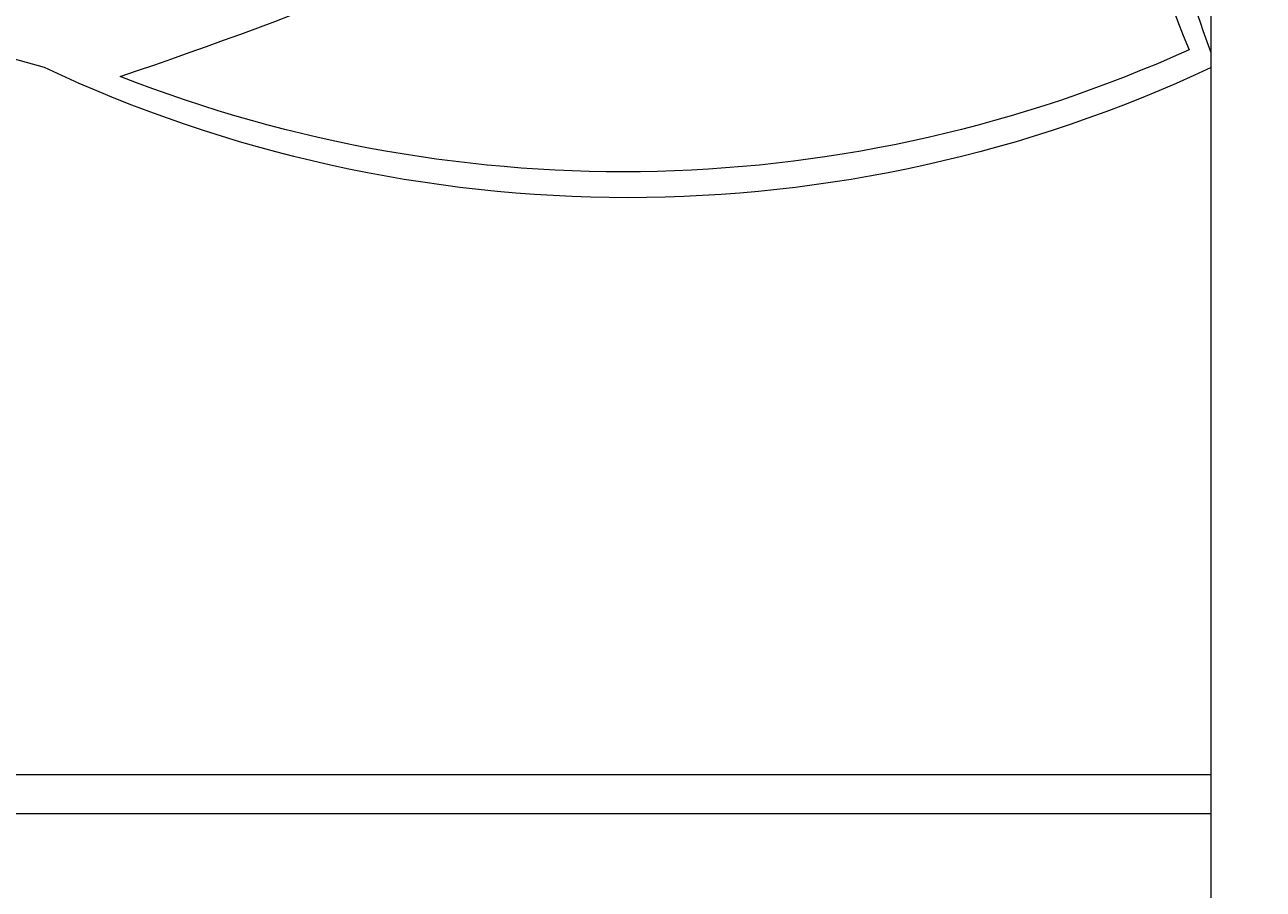
# Model space of a CAD drawing. Units: inches. Extents: x -61 to 1599, y -1316 to 257.
# Tile 38 of 204: x 134 to 171, y -763 to -738. Entities that reach past the tile are written whole.
import ezdxf

# ---------------------------------------------------------------- set-up
doc = ezdxf.new("R2010")
doc.units = ezdxf.units.IN
doc.header["$MEASUREMENT"] = 0
doc.layers.add('A-ANNO-DIMS', color=2, linetype='Continuous', lineweight=18)
doc.layers.add('FURNITURE', color=83, linetype='Continuous', lineweight=18)
doc.styles.get("Standard").update_dxf_attribs({"font": 'arial.ttf'})
doc.dimstyles.get("Standard").update_dxf_attribs({"dimtxt": 0.18, "dimasz": 0.18, "dimexe": 0.18, "dimexo": 0.0625, "dimgap": 0.09, "dimtad": 0, "dimtih": 1, "dimtoh": 1, "dimdec": 0, "dimzin": 0, "dimdsep": 46, "dimlunit": 3, "dimtxsty": 'Standard', "dimcen": 0.09, "dimadec": 0, "dimazin": 0, "dimtfac": 1, "dimtdec": 0, "dimtofl": 0, "dimtmove": 0, "dimatfit": 3, "dimfxl": 1, "dimtolj": 1, "dimtzin": 0, "dimarcsym": 0})

# ---------------------------------------------------------------- blocks, each defined once
blk = doc.blocks.new('BED-DOUBLE')
for p, q in [((1.272, 20.467), (70.263, 20.467)), ((1.272, 19.317), (70.263, 19.317))]:
    blk.add_line(p, q)
for points in [[(1.272, 88.537), (1.272, 3.449, 0.414214), (4.722, 0), (66.813, 0, 0.414214), (70.263, 3.449), (70.263, 88.537, 0.414214), (66.813, 91.987), (4.722, 91.987, 0.414214)], [(38.01, 41.126, 0.064396), (68.933, 56.181, 0.181766), (69.614, 41.916, -0.202767)]]:
    blk.add_lwpolyline(points, format="xyb", close=True)
blk.add_lwpolyline([(70.263, 41.387, -0.22309), (35.767, 41.387, 0.142156), (1.272, 41.387)], format="xyb")
for points, weights, knots in [([(70.263, 41.825), (68.018, 47.029), (68.018, 52.696), (70.263, 57.9), (69.1, 60.328), (66.924, 64.874), (70.854, 72.444), (64.929, 79.65), (71.186, 84.991), (70.014, 87.727), (69.253, 88.741)], [1, 0.945466318698, 0.945466318698, 1, 1, 1, 1, 1, 1, 1, 1], [0, 0, 0, 0, 0.814571, 0.814571, 0.814571, 7.464247, 13.266353, 20.788537, 26.138745, 29.321895, 29.321895, 29.321895, 29.321895]), ([(70.263, 57.9), (59.862, 50.943), (48.595, 45.5), (36.681, 41.677), (36.463, 41.771), (36.247, 41.868), (36.032, 41.966), (24.597, 45.284), (12.692, 45.258), (1.272, 41.889), (2.723, 44.9), (5.745, 51.172), (0.137, 60.702), (6.828, 69.972), (0.109, 77.787), (4.354, 84.383), (5.398, 86.876)], [1, 0.993520320424, 0.993520320424, 1, 0.99997444972, 0.99997444972, 1, 0.973174868659, 0.973174868659, 1, 1, 1, 1, 1, 1, 1, 1], [0, 0, 0, 0, 0.279074, 0.279074, 0.279074, 0.296584, 0.296584, 0.296584, 0.865868, 0.865868, 0.865868, 9.142578, 18.107734, 25.769226, 34.110801, 40.441511, 40.441511, 40.441511, 40.441511])]:
    blk.add_rational_spline(points, weights, degree=3, knots=knots)
blk = doc.blocks.new('*D687')
at = {"layer": 'A-ANNO-DIMS', "color": 0, "lineweight": -2, "transparency": 16777216}
for p, q in [((289.418, 181.677), (-61.077, 181.677)), ((-60.897, 181.497), (-60.897, -528.952)), ((-60.897, -1239.765), (-60.897, -529.316)), ((319.64, -1239.945), (-61.077, -1239.945))]:
    blk.add_line(p, q, dxfattribs=at)
at = {"layer": 'A-ANNO-DIMS', "color": 0, "transparency": 16777216}
for points in [[(-60.927, 181.497), (-60.867, 181.497), (-60.897, 181.677)], [(-60.927, -1239.765), (-60.867, -1239.765), (-60.897, -1239.945)]]:
    blk.add_solid(points, dxfattribs=at)
at = {"layer": 'DEFPOINTS', "color": 0, "transparency": 16777216}
for p in [(289.481, 181.677), (-60.897, -1239.945), (319.703, -1239.945)]:
    blk.add_point(p, dxfattribs=at)
at = {"layer": 'A-ANNO-DIMS', "color": 0, "transparency": 16777216, "insert": (-60.897, -529.134), "char_height": 0.18, "attachment_point": 5}
blk.add_mtext('\\A1;1421.6', dxfattribs=at)

msp = doc.modelspace()

# ---------------------------------------------------------------- block references
at = {"layer": 'FURNITURE'}
msp.add_blockref('BED-DOUBLE', (98.977, -780.4187), dxfattribs=at)

# ---------------------------------------------------------------- dimensions: what is measured, and where the dimension line sits
at = {"layer": 'A-ANNO-DIMS'}
dim = msp.add_linear_dim(base=(-60.8972, -1239.9446), p1=(289.4807, 181.6771), p2=(319.7028, -1239.9446), angle=90, dimstyle='Standard', override={"dimdec": 1, "dimlfac": 1, "dimrnd": 0, "dimzin": 0, "dimdsep": 46, "dimlunit": 2}, dxfattribs=at)
dim.commit()
dim.dimension.update_dxf_attribs({"geometry": '*D687', "text_midpoint": (-60.8972, -529.1337)})

doc.saveas('drawing.dxf')
